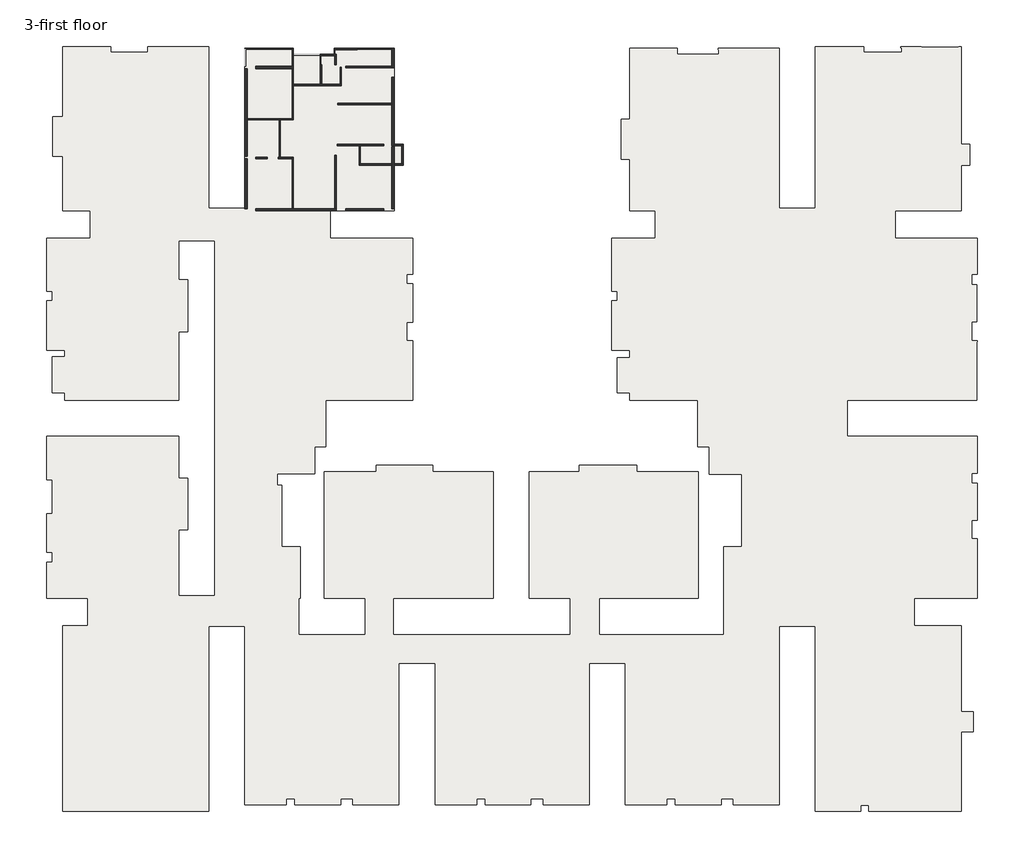
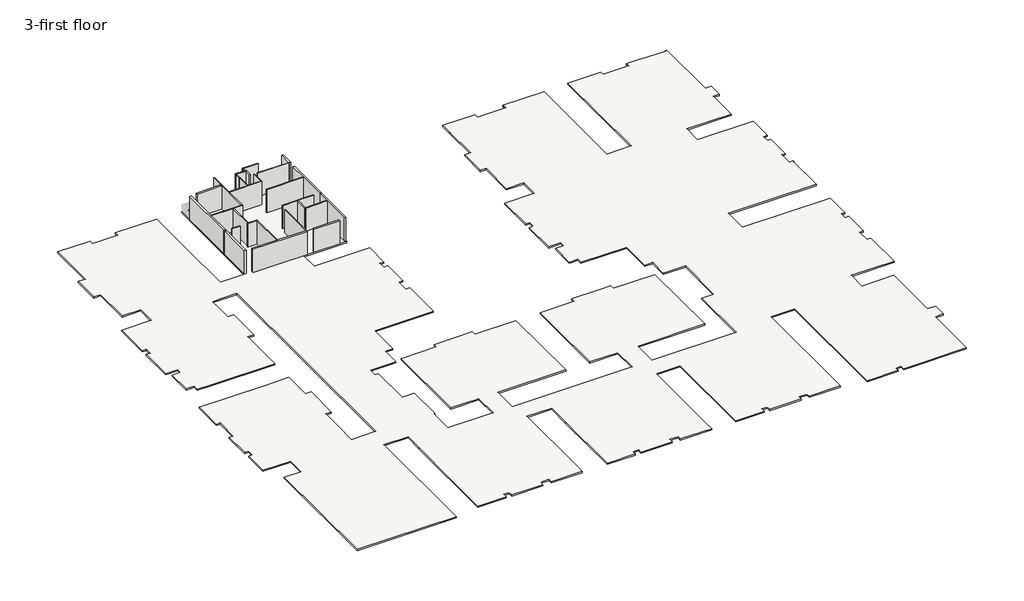
# One storey, part 1 of 2: 32 walls, 1 slab.
"""IFC4 building model written with IfcOpenShell, lengths in millimetres."""

from ifc_helpers import new_model, si_unit, frame, origin, place, context, project, spatial, polyline, outline, extrude, faceted_brep, element, save

model = new_model("IFC4")

# Units and contexts
model_context = context("Model", 3, world=origin())
ifc_project = project(units=[si_unit("LENGTHUNIT", "METRE", prefix="MILLI")], contexts=[model_context])

# Site, building, storey
site = spatial("IfcSite", under=ifc_project)
building = spatial("IfcBuilding", under=site)
storey = spatial("IfcBuildingStorey", under=building, Name="3-first floor", Elevation=3505.2)

# Slab
placement = place(None, origin())
element("IfcSlab", 1, ObjectType="6\" floor", at=placement, inside=storey, context=model_context, shape_type="SweptSolid", body=[
    extrude(outline(polyline([(-40067.5946761, 34417.793059), (-40067.5946761, 36703.793059), (-42359.0159175, 36703.793059), (-42359.0159175, 41288.4930592), (-43200.0473754, 41288.4930592), (-43200.0473754, 44641.2930588), (-42359.0159175, 44641.2930588), (-42359.0159175, 50522.1625405), (-38355.6844598, 50522.1625405), (-38355.6844598, 50026.0999818), (-35221.6159175, 50026.0999818), (-35221.6159175, 50522.1625405), (-30090.8159175, 50522.1625405), (-30090.8159175, 44272.6043046), (-30090.8159175, 36920.6122854), (-27080.9159175, 36920.6122854), (-27080.9159175, 50369.7625405), (-23004.2159175, 50369.7625405), (-23004.2159175, 49873.6841178), (-19562.5159175, 49873.6841178), (-19562.5159175, 50369.7625405), (-14510.7473752, 50369.7625405), (-14510.7473752, 42291.793059), (-13786.847376, 42291.793059), (-13786.847376, 40564.593059), (-14510.7473752, 40564.593059), (-14510.7473752, 39345.393059), (-14510.7473752, 36703.793059), (-19901.4109088, 36703.793059), (-19901.4109088, 34417.793059), (-12985.9778949, 34417.793059), (-12985.9778949, 31382.4930587), (-13482.0473762, 31382.4930587), (-13482.0473762, 30582.3930587), (-12985.9778949, 30582.3930587), (-12985.9778949, 27342.8846057), (-13482.047376, 27342.8846057), (-13482.047376, 25819.8930592), (-12985.9778949, 25819.8930592), (-12985.9778949, 20790.6930592), (-20261.0159173, 20790.6930592), (-20261.0159173, 16904.4930621), (-21213.5159173, 16904.4930621), (-21213.5159173, 14605.7930651), (-24363.1159173, 14605.7930651), (-24363.1159173, 13640.5930617), (-23956.7159173, 13640.5930617), (-23956.7159173, 8484.3930618), (-22432.7159173, 8484.3930618), (-22432.7159173, 4153.6930617), (-22552.879451, 4153.6930617), (-22552.879451, 1105.693062), (-16952.179451, 1105.693062), (-16952.179451, 4153.693062), (-20419.279451, 4153.693062), (-20419.279451, 14808.993062), (-16050.479451, 14808.993062), (-16050.479451, 15342.393062), (-11287.979451, 15342.393062), (-11287.979451, 14808.993062), (-6207.979451, 14808.993062), (-6207.979451, 4153.693062), (-14589.979451, 4153.693062), (-14589.979451, 1105.693062), (269.020549, 1105.693062), (269.020549, 4153.693062), (-3198.079451, 4153.693062), (-3198.079451, 11358.3599187), (-3198.079451, 14808.993062), (56.8139168, 14808.993062), (1031.020549, 14808.993062), (1031.020549, 15342.393062), (4447.320549, 15342.393062), (5844.320549, 15342.393062), (5844.320549, 14808.993062), (11013.220549, 14808.993062), (11013.220549, 4153.693062), (2707.420549, 4153.693062), (2707.420549, 1105.693062), (13149.6520067, 1105.693062), (13149.6520067, 8509.7930618), (14673.6520067, 8509.7930618), (14673.6520067, 14580.393062), (11930.4520067, 14580.393062), (11930.4520067, 16904.493062), (10977.9520067, 16904.493062), (10977.9520067, 20790.6930623), (5260.120549, 20790.6930623), (5260.120549, 21438.3930622), (4231.4205485, 21438.3930622), (4231.4205485, 24372.093062), (5260.120549, 24372.093062), (5260.120549, 25007.093059), (3735.3510676, 25007.093059), (3735.3510676, 29155.9725232), (4231.4205489, 29155.9725232), (4231.4205489, 29972.793059), (3735.3510673, 29972.793059), (3735.3510673, 34417.793062), (7406.6788707, 34417.793062), (7406.6788707, 36703.793062), (5262.3642609, 36703.793062), (5262.3642609, 41072.593062), (4538.4642607, 41072.593062), (4538.4642607, 44425.393062), (5262.3642609, 44425.393062), (5262.3642609, 48850.8834653), (5262.3642609, 50369.7625405), (9260.0328033, 50369.7625405), (9260.0328033, 49861.0033239), (12752.53262, 49861.0033239), (12752.53262, 50255.4613897), (12701.7328035, 50255.4613897), (12701.7328035, 50369.7625391), (17833.6918765, 50369.7625391), (17833.6918765, 36920.6122884), (20843.020549, 36920.6122884), (20843.020549, 50522.1625435), (24922.5520067, 50522.1625435), (24922.5520067, 50026.0682305), (28107.4205486, 50026.0682305), (28107.4205486, 50407.8625436), (28056.620549, 50407.8625436), (28056.620549, 50522.1625436), (29758.420549, 50522.1625436), (29758.420549, 50464.6477108), (32908.0205485, 50464.6477108), (32908.0205485, 50522.1625436), (33111.220549, 50522.1625436), (33111.220549, 42291.793059), (33835.1205481, 42291.793059), (33835.1205481, 40564.593059), (33111.220549, 40564.593059), (33111.220549, 36703.793062), (27583.8962522, 36703.793062), (27583.8962522, 34417.793062), (34483.5900291, 34417.793062), (34483.5900291, 31369.7930587), (33987.5205478, 31369.7930587), (33987.5205478, 30518.8930587), (34420.0900291, 30518.8930587), (34420.0900291, 27393.6846085), (33987.520548, 27393.6846085), (33987.520548, 25819.8930599), (34483.5900268, 25819.8930599), (34483.5900268, 25718.293062), (34420.0900291, 25718.293062), (34420.0900291, 20790.6930621), (23560.820549, 20790.6930621), (23560.820549, 17780.7930626), (34470.8900301, 17780.7930626), (34470.8900301, 14669.2930621), (33987.5205488, 14669.2930621), (33987.5205488, 13831.5086417), (34470.8900301, 13831.5086417), (34470.8900301, 10719.5930626), (33987.520549, 10719.5930626), (33987.520549, 9144.7930626), (34483.5900287, 9144.7930626), (34483.5900287, 4153.6930626), (29171.7035804, 4153.6930626), (29171.7035804, 1867.6930615), (33111.220549, 1867.6930615), (33111.220549, -4382.5255151), (33111.220549, -5358.6069385), (34139.9205493, -5358.6069385), (34139.9205493, -7035.0069385), (33111.220549, -7035.0069385), (33111.220549, -12216.6069385), (33111.220549, -13741.3764277), (25342.0873109, -13741.3764277), (25342.0873109, -13245.3069411), (24664.0464127, -13245.3069411), (24664.0464127, -13741.3764224), (20843.020549, -13741.3764224), (20843.020549, 1791.493062), (17833.120549, 1791.493062), (17833.1205601, -12469.7116346), (17833.1205601, -13181.806941), (13972.320549, -13181.806941), (13972.320549, -12686.5069412), (12968.4328031, -12686.5069412), (12968.4328031, -13181.806941), (9079.9890911, -13181.806941), (9079.9890911, -12686.5069411), (8371.620549, -12686.5069411), (8371.620549, -13181.806941), (4879.120549, -13181.806941), (4879.120549, -1281.906938), (1869.220549, -1281.906938), (1869.2205601, -11657.8069405), (1869.2205601, -13181.806941), (-1991.579451, -13181.806941), (-1991.579451, -12686.5069412), (-3032.979451, -12686.5069412), (-3032.979451, -13181.806941), (-6883.9109089, -13181.806941), (-6883.9109089, -12686.5069411), (-7592.2794511, -12686.5069411), (-7592.2794511, -13181.806941), (-11084.779451, -13181.806941), (-11084.779451, -4364.4278939), (-11084.779451, -1281.906938), (-14132.779451, -1281.906938), (-14132.7794399, -11657.8069405), (-14132.7794399, -13181.806941), (-17993.579451, -13181.806941), (-17993.579451, -12686.5069412), (-19034.979451, -12686.5069412), (-19034.979451, -13181.806941), (-22885.9109089, -13181.806941), (-22885.9109089, -12686.5069411), (-23594.279451, -12686.5069411), (-23594.279451, -13181.806941), (-27086.779451, -13181.806941), (-27086.779451, -630.8240429), (-27086.779451, 1791.493062), (-30096.679451, 1791.493062), (-30096.679451, -13741.3764224), (-42359.0159175, -13741.3764224), (-42359.0159175, 1867.6930615), (-40274.4710752, 1867.6930615), (-40274.4710752, 4153.6930619), (-43737.2489325, 4153.6930619), (-43737.2489325, 7188.9930625), (-43244.0109091, 7188.9930625), (-43244.0109091, 8035.7406725), (-43740.0803903, 8035.7406725), (-43740.0803903, 11278.3930621), (-43244.0109091, 11278.3930621), (-43244.0109091, 14123.1930621), (-43737.2489325, 14123.1930621), (-43737.2489325, 17780.7930616), (-35451.4646582, 17780.7930627), (-32611.279451, 17780.7930627), (-32611.279451, 14237.4930616), (-31890.2109088, 14237.4930616), (-31890.2109088, 9905.7846088), (-32611.2794515, 9905.7846088), (-32611.279451, 7112.7930625), (-32611.279451, 4382.2930626), (-29601.379451, 4382.2930626), (-29601.379451, 34189.193059), (-32614.110909, 34189.193059), (-32614.110909, 32865.9503102), (-32614.110909, 30913.6015126), (-31890.210909, 30913.6015126), (-31890.210909, 27445.4930592), (-31890.210909, 26569.1930592), (-32614.110909, 26569.1930592), (-32614.110909, 20790.6930591), (-40664.490635, 20790.6930591), (-42212.479451, 20790.6930591), (-42212.479451, 21438.393059), (-43244.0109092, 21438.393059), (-43244.0109092, 24435.5930825), (-42215.3109116, 24435.5930825), (-42215.3109116, 24994.393059), (-43740.0803903, 24994.393059), (-43740.0803903, 29172.693059), (-43244.0109091, 29172.693059), (-43244.0109091, 29972.793059), (-43740.0803903, 29972.793059), (-43740.0803903, 34417.793059), (-40067.5946761, 34417.793059)])), frame((0.0, 0.0, 3352.8), z_axis=(0.0, 0.0, 1.0), x_axis=(1.0, 0.0, 0.0)), (0.0, 0.0, 1.0), 152.4),
])

# Walls
element("IfcWall", 2, ObjectType="1\"", at=placement, inside=storey, context=model_context, shape_type="SweptSolid", body=[
    extrude(outline(polyline([(-20680.9533155, 49759.3844575), (-20680.9533155, 49003.2834458), (-20721.5933155, 49003.2834458), (-20721.5933155, 49759.3844575), (-20680.9533155, 49759.3844575)])), frame((0.0, 0.0, 3505.2), z_axis=(0.0, 0.0, 1.0), x_axis=(1.0, 0.0, 0.0)), (0.0, 0.0, 1.0), 3048.0),
])
element("IfcWall", 3, ObjectType="2.5\"", at=placement, inside=storey, context=model_context, shape_type="SweptSolid", body=[
    extrude(outline(polyline([(-19562.5159175, 49873.6844575), (-19562.5159175, 50255.4625405), (-19504.0959175, 50255.4625405), (-19504.0959175, 49873.6844575), (-19562.5159175, 49873.6844575)])), frame((0.0, 0.0, 3505.2), z_axis=(0.0, 0.0, 1.0), x_axis=(1.0, 0.0, 0.0)), (0.0, 0.0, 1.0), 3048.0),
])
element("IfcWall", 4, ObjectType="4\" wall", at=placement, inside=storey, context=model_context, shape_type="Brep", body=[
    faceted_brep([(-26877.7159175, 44361.8930595, 3505.2), (-24198.0159175, 44361.8930595, 3505.2), (-24096.4159175, 44361.8930595, 3505.2), (-23004.2159175, 44361.8930595, 3505.2), (-23004.2159175, 44361.8930595, 6553.2), (-24096.4159175, 44361.8930595, 6553.2), (-24198.0159175, 44361.8930595, 6553.2), (-26877.7159175, 44361.8930595, 6553.2), (-26877.7159175, 44463.4930595, 3505.2), (-26877.7159175, 44463.4930595, 6553.2), (-23105.8159175, 44463.4930595, 6553.2), (-23004.2159175, 44463.4930595, 6553.2), (-23004.2159175, 44463.4930595, 3505.2), (-23105.8159175, 44463.4930595, 3505.2)], [[[0, 1, 2, 3, 4, 5, 6, 7]], [[8, 9, 10, 11, 12, 13]], [[3, 2, 1, 0, 8, 13, 12]], [[7, 6, 5, 4, 11, 10, 9]], [[0, 7, 9, 8]], [[4, 3, 12, 11]]]),
])
element("IfcWall", 5, ObjectType="4\" wall", at=placement, inside=storey, context=model_context, shape_type="Brep", body=[
    faceted_brep([(-23004.2159175, 44463.4930595, 3505.2), (-23004.2159175, 47237.9834458, 3505.2), (-23004.2159175, 47339.5834458, 3505.2), (-23004.2159175, 48647.683515, 3505.2), (-23004.2159175, 48647.683515, 6553.2), (-23004.2159175, 47339.5834458, 6553.2), (-23004.2159175, 47237.9834458, 6553.2), (-23004.2159175, 44463.4930595, 6553.2), (-23105.8159175, 44463.4930595, 3505.2), (-23105.8159175, 44463.4930595, 6553.2), (-23105.8159175, 48647.683515, 6553.2), (-23105.8159175, 48647.683515, 3505.2)], [[[0, 1, 2, 3, 4, 5, 6, 7]], [[8, 9, 10, 11]], [[3, 2, 1, 0, 8, 11]], [[7, 6, 5, 4, 10, 9]], [[0, 7, 9, 8]], [[4, 3, 11, 10]]]),
])
element("IfcWall", 6, ObjectType="4\" wall", at=placement, inside=storey, context=model_context, shape_type="Brep", body=[
    faceted_brep([(-20731.7533155, 49003.2834458, 3505.2), (-20731.7533155, 47339.5834458, 3505.2), (-20731.7533155, 47339.5834458, 6553.2), (-20731.7533155, 49003.2834458, 6553.2), (-20630.1533155, 49003.2834458, 3505.2), (-20630.1533155, 49003.2834458, 6553.2), (-20630.1533155, 47339.5834458, 6553.2), (-20630.1533155, 47339.5834458, 3505.2), (-20721.5933155, 49003.2834458, 3505.2), (-20680.9533155, 49003.2834458, 3505.2), (-20680.9533155, 49003.2834458, 6553.2), (-20721.5933155, 49003.2834458, 6553.2)], [[[0, 1, 2, 3]], [[4, 5, 6, 7]], [[1, 0, 8, 9, 4, 7]], [[3, 2, 6, 5, 10, 11]], [[0, 3, 11, 10, 5, 4, 9, 8]], [[2, 1, 7, 6]]]),
])
element("IfcWall", 7, ObjectType="4\" wall", at=placement, inside=storey, context=model_context, shape_type="Brep", body=[
    faceted_brep([(-23004.2159175, 47237.9834458, 3505.2), (-18955.7473752, 47237.9834458, 3505.2), (-18955.7473752, 47237.9834458, 6553.2), (-23004.2159175, 47237.9834458, 6553.2), (-23004.2159175, 47339.5834458, 3505.2), (-23004.2159175, 47339.5834458, 6553.2), (-20731.7533155, 47339.5834458, 6553.2), (-20630.1533155, 47339.5834458, 6553.2), (-19057.3473752, 47339.5834458, 6553.2), (-18955.7473752, 47339.5834458, 6553.2), (-18955.7473752, 47339.5834458, 3505.2), (-19057.3473752, 47339.5834458, 3505.2), (-20630.1533155, 47339.5834458, 3505.2), (-20731.7533155, 47339.5834458, 3505.2)], [[[0, 1, 2, 3]], [[4, 5, 6, 7, 8, 9, 10, 11, 12, 13]], [[1, 0, 4, 13, 12, 11, 10]], [[3, 2, 9, 8, 7, 6, 5]], [[2, 1, 10, 9]], [[0, 3, 5, 4]]]),
])
element("IfcWall", 8, ObjectType="4\" wall", at=placement, inside=storey, context=model_context, shape_type="SweptSolid", body=[
    extrude(outline(polyline([(-18955.7473752, 48800.0834491), (-18955.7473752, 47339.5834458), (-19057.3473752, 47339.5834458), (-19057.3473752, 48800.0834491), (-18955.7473752, 48800.0834491)])), frame((0.0, 0.0, 3505.2), z_axis=(0.0, 0.0, 1.0), x_axis=(1.0, 0.0, 0.0)), (0.0, 0.0, 1.0), 3048.0),
])
element("IfcWall", 9, ObjectType="4\" wall", at=placement, inside=storey, context=model_context, shape_type="SweptSolid", body=[
    extrude(outline(polyline([(-18587.4473751, 48850.8834491), (-14713.9473752, 48850.8834491), (-14713.9473752, 48749.2834491), (-18587.4473751, 48749.2834491), (-18587.4473751, 48850.8834491)])), frame((0.0, 0.0, 3505.2), z_axis=(0.0, 0.0, 1.0), x_axis=(1.0, 0.0, 0.0)), (0.0, 0.0, 1.0), 3048.0),
])
element("IfcWall", 10, ObjectType="4\" wall", at=placement, inside=storey, context=model_context, shape_type="SweptSolid", body=[
    extrude(outline(polyline([(-19285.9473752, 45746.193059), (-14713.9473752, 45746.193059), (-14713.9473752, 45644.593059), (-19285.9473752, 45644.593059), (-19285.9473752, 45746.193059)])), frame((0.0, 0.0, 3505.2), z_axis=(0.0, 0.0, 1.0), x_axis=(1.0, 0.0, 0.0)), (0.0, 0.0, 1.0), 3048.0),
])
element("IfcWall", 11, ObjectType="4\" wall", at=placement, inside=storey, context=model_context, shape_type="Brep", body=[
    faceted_brep([(-15425.1473762, 42291.793059, 3505.2), (-19298.6473752, 42291.793059, 3505.2), (-19298.6473752, 42291.793059, 6553.2), (-15425.1473762, 42291.793059, 6553.2), (-15425.1473762, 42190.193059, 3505.2), (-15425.1473762, 42190.193059, 6553.2), (-17380.9473752, 42190.193059, 6553.2), (-17482.5473752, 42190.193059, 6553.2), (-19298.6473752, 42190.193059, 6553.2), (-19298.6473752, 42190.193059, 3505.2), (-17482.5473752, 42190.193059, 3505.2), (-17380.9473752, 42190.193059, 3505.2)], [[[0, 1, 2, 3]], [[4, 5, 6, 7, 8, 9, 10, 11]], [[1, 0, 4, 11, 10, 9]], [[2, 1, 9, 8]], [[3, 2, 8, 7, 6, 5]], [[0, 3, 5, 4]]]),
])
element("IfcWall", 12, ObjectType="4\" wall", at=placement, inside=storey, context=model_context, shape_type="SweptSolid", body=[
    extrude(outline(polyline([(-19501.8473752, 36906.993059), (-19501.8473752, 41377.3930622), (-19400.2473752, 41377.3930622), (-19400.2473752, 36906.993059), (-19501.8473752, 36906.993059)])), frame((0.0, 0.0, 3505.2), z_axis=(0.0, 0.0, 1.0), x_axis=(1.0, 0.0, 0.0)), (0.0, 0.0, 1.0), 3048.0),
])
element("IfcWall", 13, ObjectType="4\" wall", at=placement, inside=storey, context=model_context, shape_type="Brep", body=[
    faceted_brep([(-17482.5473752, 42190.193059, 3505.2), (-17482.5473752, 40564.593059, 3505.2), (-17482.5473752, 40564.593059, 6553.2), (-17482.5473752, 42190.193059, 6553.2), (-17380.9473752, 42190.193059, 3505.2), (-17380.9473752, 42190.193059, 6553.2), (-17380.9473752, 40666.193059, 6553.2), (-17380.9473752, 40564.593059, 6553.2), (-17380.9473752, 40564.593059, 3505.2), (-17380.9473752, 40666.193059, 3505.2)], [[[0, 1, 2, 3]], [[4, 5, 6, 7, 8, 9]], [[1, 0, 4, 9, 8]], [[3, 2, 7, 6, 5]], [[0, 3, 5, 4]], [[2, 1, 8, 7]]]),
])
element("IfcWall", 14, ObjectType="4\" wall", at=placement, inside=storey, context=model_context, shape_type="SweptSolid", body=[
    extrude(outline(polyline([(-14713.9473762, 40564.593059), (-17380.9473752, 40564.593059), (-17380.9473752, 40666.193059), (-14713.9473762, 40666.193059), (-14713.9473762, 40564.593059)])), frame((0.0, 0.0, 3505.2), z_axis=(0.0, 0.0, 1.0), x_axis=(1.0, 0.0, 0.0)), (0.0, 0.0, 1.0), 3048.0),
])
element("IfcWall", 15, ObjectType="4\" wall", at=placement, inside=storey, context=model_context, shape_type="Brep", body=[
    faceted_brep([(-14510.7473762, 40564.593059, 3505.2), (-13786.847376, 40564.593059, 3505.2), (-13786.847376, 40564.593059, 5334.0), (-14510.7473762, 40564.593059, 5334.0), (-14510.7473762, 40666.193059, 3505.2), (-14510.7473762, 40666.193059, 5334.0), (-13888.447376, 40666.193059, 5334.0), (-13786.847376, 40666.193059, 5334.0), (-13786.847376, 40666.193059, 3505.2), (-13888.447376, 40666.193059, 3505.2)], [[[0, 1, 2, 3]], [[4, 5, 6, 7, 8, 9]], [[1, 0, 4, 9, 8]], [[3, 2, 7, 6, 5]], [[0, 3, 5, 4]], [[2, 1, 8, 7]]]),
])
element("IfcWall", 16, ObjectType="4\" wall", at=placement, inside=storey, context=model_context, shape_type="Brep", body=[
    faceted_brep([(-14510.7473752, 42190.193059, 3505.2), (-13888.447376, 42190.193059, 3505.2), (-13786.847376, 42190.193059, 3505.2), (-13786.847376, 42190.193059, 5334.0), (-13888.447376, 42190.193059, 5334.0), (-14510.7473752, 42190.193059, 5334.0), (-14510.7473752, 42291.793059, 3505.2), (-14510.7473752, 42291.793059, 5334.0), (-13786.847376, 42291.793059, 5334.0), (-13786.847376, 42291.793059, 3505.2)], [[[0, 1, 2, 3, 4, 5]], [[6, 7, 8, 9]], [[2, 1, 0, 6, 9]], [[5, 4, 3, 8, 7]], [[0, 5, 7, 6]], [[3, 2, 9, 8]]]),
])
element("IfcWall", 17, ObjectType="4\" wall", at=placement, inside=storey, context=model_context, shape_type="SweptSolid", body=[
    extrude(outline(polyline([(-13888.447376, 40666.193059), (-13888.447376, 42190.193059), (-13786.847376, 42190.193059), (-13786.847376, 40666.193059), (-13888.447376, 40666.193059)])), frame((0.0, 0.0, 3505.2), z_axis=(0.0, 0.0, 1.0), x_axis=(1.0, 0.0, 0.0)), (0.0, 0.0, 1.0), 1828.8),
])
element("IfcWall", 18, ObjectType="4\" wall", at=placement, inside=storey, context=model_context, shape_type="Brep", body=[
    faceted_brep([(-23004.2159175, 36906.993059, 3505.2), (-23004.2159175, 41212.293059, 3505.2), (-23004.2159175, 41212.293059, 6553.2), (-23004.2159175, 36906.993059, 6553.2), (-23105.8159175, 36906.993059, 3505.2), (-23105.8159175, 36906.993059, 6553.2), (-23105.8159175, 41110.693059, 6553.2), (-23105.8159175, 41212.293059, 6553.2), (-23105.8159175, 41212.293059, 3505.2), (-23105.8159175, 41110.693059, 3505.2)], [[[0, 1, 2, 3]], [[4, 5, 6, 7, 8, 9]], [[1, 0, 4, 9, 8]], [[3, 2, 7, 6, 5]], [[0, 3, 5, 4]], [[2, 1, 8, 7]]]),
])
element("IfcWall", 19, ObjectType="4\" wall", at=placement, inside=storey, context=model_context, shape_type="Brep", body=[
    faceted_brep([(-23105.8159175, 41212.293059, 3505.2), (-24096.4159175, 41212.293059, 3505.2), (-24198.0159175, 41212.293059, 3505.2), (-24261.5159175, 41212.293059, 3505.2), (-24261.5159175, 41212.293059, 6553.2), (-24198.0159175, 41212.293059, 6553.2), (-24096.4159175, 41212.293059, 6553.2), (-23105.8159175, 41212.293059, 6553.2), (-23105.8159175, 41110.693059, 3505.2), (-23105.8159175, 41110.693059, 6553.2), (-24261.5159175, 41110.693059, 6553.2), (-24261.5159175, 41110.693059, 3505.2)], [[[0, 1, 2, 3, 4, 5, 6, 7]], [[8, 9, 10, 11]], [[3, 2, 1, 0, 8, 11]], [[4, 3, 11, 10]], [[7, 6, 5, 4, 10, 9]], [[0, 7, 9, 8]]]),
])
element("IfcWall", 20, ObjectType="4\" wall", at=placement, inside=storey, context=model_context, shape_type="SweptSolid", body=[
    extrude(outline(polyline([(-26166.5159175, 41212.293059), (-25175.9159175, 41212.293059), (-25175.9159175, 41110.693059), (-26166.5159175, 41110.693059), (-26166.5159175, 41212.293059)])), frame((0.0, 0.0, 3505.2), z_axis=(0.0, 0.0, 1.0), x_axis=(1.0, 0.0, 0.0)), (0.0, 0.0, 1.0), 3048.0),
])
element("IfcWall", 21, ObjectType="4\" wall", at=placement, inside=storey, context=model_context, shape_type="SweptSolid", body=[
    extrude(outline(polyline([(-24096.4159175, 44361.8930595), (-24096.4159175, 41212.293059), (-24198.0159175, 41212.293059), (-24198.0159175, 44361.8930595), (-24096.4159175, 44361.8930595)])), frame((0.0, 0.0, 3505.2), z_axis=(0.0, 0.0, 1.0), x_axis=(1.0, 0.0, 0.0)), (0.0, 0.0, 1.0), 3048.0),
])
element("IfcWall", 22, ObjectType="4\" wall", at=placement, inside=storey, context=model_context, shape_type="SweptSolid", body=[
    extrude(outline(polyline([(-23105.8159175, 48850.883515), (-23105.8159175, 50369.7625405), (-23004.2159175, 50369.7625405), (-23004.2159175, 48850.883515), (-23105.8159175, 48850.883515)])), frame((0.0, 0.0, 3505.2), z_axis=(0.0, 0.0, 1.0), x_axis=(1.0, 0.0, 0.0)), (0.0, 0.0, 1.0), 3048.0),
])
element("IfcWall", 23, ObjectType="4\" wall", at=placement, inside=storey, context=model_context, shape_type="SweptSolid", body=[
    extrude(outline(polyline([(-19501.8473751, 49003.2834458), (-19501.8473751, 49759.3844575), (-19400.2473751, 49759.3844575), (-19400.2473751, 49003.2834458), (-19501.8473751, 49003.2834458)])), frame((0.0, 0.0, 3505.2), z_axis=(0.0, 0.0, 1.0), x_axis=(1.0, 0.0, 0.0)), (0.0, 0.0, 1.0), 3048.0),
])
element("IfcWall", 24, ObjectType="4.5\" wall", at=placement, inside=storey, context=model_context, shape_type="Brep", body=[
    faceted_brep([(-19400.2473751, 49873.6844575, 3505.2), (-19504.0959175, 49873.6844575, 3505.2), (-19562.5159175, 49873.6844575, 3505.2), (-20721.5933155, 49873.6844575, 3505.2), (-20721.5933155, 49873.6844575, 6553.2), (-19562.5159175, 49873.6844575, 6553.2), (-19504.0959175, 49873.6844575, 6553.2), (-19400.2473751, 49873.6844575, 6553.2), (-19400.2473751, 49759.3844575, 3505.2), (-19400.2473751, 49759.3844575, 6553.2), (-19501.8473751, 49759.3844575, 6553.2), (-20680.9533155, 49759.3844575, 6553.2), (-20721.5933155, 49759.3844575, 6553.2), (-20721.5933155, 49759.3844575, 3505.2), (-20680.9533155, 49759.3844575, 3505.2), (-19501.8473751, 49759.3844575, 3505.2)], [[[0, 1, 2, 3, 4, 5, 6, 7]], [[8, 9, 10, 11, 12, 13, 14, 15]], [[3, 2, 1, 0, 8, 15, 14, 13]], [[7, 6, 5, 4, 12, 11, 10, 9]], [[0, 7, 9, 8]], [[4, 3, 13, 12]]]),
])
element("IfcWall", 25, ObjectType="4.5\" wall", at=placement, inside=storey, context=model_context, shape_type="Brep", body=[
    faceted_brep([(-17647.6473751, 50369.7625405, 3505.2), (-19562.5159175, 50369.7625405, 3505.2), (-19562.5159175, 50369.7625405, 6553.2), (-17647.6473751, 50369.7625405, 6553.2), (-17647.6473751, 50255.4625405, 3505.2), (-17647.6473751, 50255.4625405, 6553.2), (-19504.0959175, 50255.4625405, 6553.2), (-19562.5159175, 50255.4625405, 6553.2), (-19562.5159175, 50255.4625405, 3505.2), (-19504.0959175, 50255.4625405, 3505.2)], [[[0, 1, 2, 3]], [[4, 5, 6, 7, 8, 9]], [[1, 0, 4, 9, 8]], [[3, 2, 7, 6, 5]], [[0, 3, 5, 4]], [[2, 1, 8, 7]]]),
])
element("IfcWall", 26, ObjectType="8\" wall", at=placement, inside=storey, context=model_context, shape_type="Brep", body=[
    faceted_brep([(-14713.9473752, 50369.7625405, 3505.2), (-14713.9473752, 48850.8834491, 3505.2), (-14713.9473752, 48749.2834491, 3505.2), (-14713.9473752, 48749.2834491, 6553.2), (-14713.9473752, 48850.8834491, 6553.2), (-14713.9473752, 50369.7625405, 6553.2), (-14510.7473752, 50369.7625405, 3505.2), (-14510.7473752, 50369.7625405, 6553.2), (-14510.7473752, 48850.8834491, 6553.2), (-14510.7473752, 48749.2834491, 6553.2), (-14510.7473752, 48749.2834491, 3505.2), (-14510.7473752, 48850.8834491, 3505.2)], [[[0, 1, 2, 3, 4, 5]], [[6, 7, 8, 9, 10, 11]], [[2, 1, 0, 6, 11, 10]], [[5, 4, 3, 9, 8, 7]], [[0, 5, 7, 6]], [[3, 2, 10, 9]]]),
])
element("IfcWall", 27, ObjectType="8\" wall", at=placement, inside=storey, context=model_context, shape_type="Brep", body=[
    faceted_brep([(-14713.9473752, 47936.4834491, 3505.2), (-14713.9473752, 45746.193059, 3505.2), (-14713.9473752, 45644.593059, 3505.2), (-14713.9473752, 42291.793059, 3505.2), (-14713.9473752, 42190.193059, 3505.2), (-14713.9473752, 42190.193059, 6553.2), (-14713.9473752, 42291.793059, 6553.2), (-14713.9473752, 45644.593059, 6553.2), (-14713.9473752, 45746.193059, 6553.2), (-14713.9473752, 47936.4834491, 6553.2), (-14510.7473752, 47936.4834491, 3505.2), (-14510.7473752, 47936.4834491, 6553.2), (-14510.7473752, 42190.193059, 6553.2), (-14510.7473752, 42190.193059, 5334.0), (-14510.7473752, 42190.193059, 3505.2), (-14510.7473752, 42291.793059, 3505.2)], [[[0, 1, 2, 3, 4, 5, 6, 7, 8, 9]], [[10, 11, 12, 13, 14, 15]], [[4, 3, 2, 1, 0, 10, 15, 14]], [[9, 8, 7, 6, 5, 12, 11]], [[0, 9, 11, 10]], [[5, 4, 14, 13, 12]]]),
])
element("IfcWall", 28, ObjectType="8\" wall", at=placement, inside=storey, context=model_context, shape_type="Brep", body=[
    faceted_brep([(-26166.5159189, 48647.683515, 3505.2), (-23105.8159175, 48647.683515, 3505.2), (-23004.2159175, 48647.683515, 3505.2), (-23004.2159175, 48647.683515, 6553.2), (-23105.8159175, 48647.683515, 6553.2), (-26166.5159189, 48647.683515, 6553.2), (-26166.5159189, 48850.883515, 3505.2), (-26166.5159189, 48850.883515, 6553.2), (-23105.8159175, 48850.883515, 6553.2), (-23004.2159175, 48850.883515, 6553.2), (-23004.2159175, 48850.883515, 3505.2), (-23105.8159175, 48850.883515, 3505.2)], [[[0, 1, 2, 3, 4, 5]], [[6, 7, 8, 9, 10, 11]], [[2, 1, 0, 6, 11, 10]], [[5, 4, 3, 9, 8, 7]], [[0, 5, 7, 6]], [[3, 2, 10, 9]]]),
])
element("IfcWall", 29, ObjectType="8\" wall", at=placement, inside=storey, context=model_context, shape_type="Brep", body=[
    faceted_brep([(-27080.9159175, 48647.683515, 3505.2), (-27080.9159175, 41313.8930626, 3505.2), (-27080.9159175, 41313.8930626, 6553.2), (-27080.9159175, 48647.683515, 6553.2), (-26877.7159175, 48647.683515, 3505.2), (-26877.7159175, 48647.683515, 6553.2), (-26877.7159175, 44463.4930595, 6553.2), (-26877.7159175, 44361.8930595, 6553.2), (-26877.7159175, 41313.8930626, 6553.2), (-26877.7159175, 41313.8930626, 3505.2), (-26877.7159175, 44361.8930595, 3505.2), (-26877.7159175, 44463.4930595, 3505.2)], [[[0, 1, 2, 3]], [[4, 5, 6, 7, 8, 9, 10, 11]], [[1, 0, 4, 11, 10, 9]], [[2, 1, 9, 8]], [[3, 2, 8, 7, 6, 5]], [[0, 3, 5, 4]]]),
])
element("IfcWall", 30, ObjectType="8\" wall", at=placement, inside=storey, context=model_context, shape_type="SweptSolid", body=[
    extrude(outline(polyline([(-27080.9159175, 36906.993059), (-27080.9159175, 41110.6930626), (-26877.7159175, 41110.6930626), (-26877.7159175, 36906.993059), (-27080.9159175, 36906.993059)])), frame((0.0, 0.0, 3505.2), z_axis=(0.0, 0.0, 1.0), x_axis=(1.0, 0.0, 0.0)), (0.0, 0.0, 1.0), 3048.0),
])
element("IfcWall", 31, ObjectType="8\" wall", at=placement, inside=storey, context=model_context, shape_type="Brep", body=[
    faceted_brep([(-26166.5159175, 36703.793059, 3505.2), (-19501.8473751, 36703.793059, 3505.2), (-19400.2473752, 36703.793059, 3505.2), (-19400.2473752, 36703.793059, 6553.2), (-19501.8473751, 36703.793059, 6553.2), (-26166.5159175, 36703.793059, 6553.2), (-26166.5159175, 36906.993059, 3505.2), (-26166.5159175, 36906.993059, 6553.2), (-23105.8159175, 36906.993059, 6553.2), (-23004.2159175, 36906.993059, 6553.2), (-19501.8473752, 36906.993059, 6553.2), (-19400.2473752, 36906.993059, 6553.2), (-19400.2473752, 36906.993059, 3505.2), (-19501.8473752, 36906.993059, 3505.2), (-23004.2159175, 36906.993059, 3505.2), (-23105.8159175, 36906.993059, 3505.2)], [[[0, 1, 2, 3, 4, 5]], [[6, 7, 8, 9, 10, 11, 12, 13, 14, 15]], [[2, 1, 0, 6, 15, 14, 13, 12]], [[5, 4, 3, 11, 10, 9, 8, 7]], [[0, 5, 7, 6]], [[3, 2, 12, 11]]]),
])
element("IfcWall", 32, ObjectType="8\" wall", at=placement, inside=storey, context=model_context, shape_type="Brep", body=[
    faceted_brep([(-14713.9473762, 42088.593059, 3505.2), (-14713.9473762, 40666.193059, 3505.2), (-14713.9473762, 40564.593059, 3505.2), (-14713.9473762, 36906.993059, 3505.2), (-14713.9473762, 36906.993059, 6553.2), (-14713.9473762, 40564.593059, 6553.2), (-14713.9473762, 40666.193059, 6553.2), (-14713.9473762, 42088.593059, 6553.2), (-14510.7473762, 42088.593059, 3505.2), (-14510.7473762, 42088.593059, 6553.2), (-14510.7473762, 36906.993059, 6553.2), (-14510.7473762, 36906.993059, 3505.2), (-14510.7473762, 40564.593059, 3505.2), (-14510.7473762, 40666.193059, 3505.2)], [[[0, 1, 2, 3, 4, 5, 6, 7]], [[8, 9, 10, 11, 12, 13]], [[3, 2, 1, 0, 8, 13, 12, 11]], [[4, 3, 11, 10]], [[7, 6, 5, 4, 10, 9]], [[0, 7, 9, 8]]]),
])
element("IfcWall", 33, ObjectType="8\" wall", at=placement, inside=storey, context=model_context, shape_type="SweptSolid", body=[
    extrude(outline(polyline([(-18587.4473751, 36906.993059), (-15425.1473752, 36906.993059), (-15425.1473752, 36703.793059), (-18587.4473751, 36703.793059), (-18587.4473751, 36906.993059)])), frame((0.0, 0.0, 3505.2), z_axis=(0.0, 0.0, 1.0), x_axis=(1.0, 0.0, 0.0)), (0.0, 0.0, 1.0), 3048.0),
])

save(model, "model.ifc")

# Revit data of these elements
# Type "6\" floor"
#   Assembly Code = "B1010"
#   Function = 0
#   Layers, outside or top first: 0' - 6" no material (function 1)
# Type "1\""
#   Assembly Code = "B2010"
#   Layers, outside or top first: 0' - 1 77/128" "00-8\" wall" (function 1)
# Type "2.5\""
#   Assembly Code = "B2010"
#   Layers, outside or top first: 0' - 2 77/256" "00-8\" wall" (function 1)
# Type "4\" wall"
#   Assembly Code = "B2010"
#   Layers, outside or top first: 0' - 4" "00-8\" wall" (function 1)
# Type "4.5\" wall"
#   Assembly Code = "B2010"
#   Layers, outside or top first: 0' - 4 1/2" "00-8\" wall" (function 1)
# Type "8\" wall"
#   Assembly Code = "B2010"
#   Layers, outside or top first: 0' - 8" "00-8\" wall" (function 1)
# Element 1 (IfcSlab, "6\" floor")
#   built-in parameter 1001955 = -1.5708 (stored number, unit not read)
#   Height Offset From Level = 0' - 0"
#   Phase Created = New Construction
#   Materials on its faces: "Default Floor"
# Element 2 (IfcWall, "1\"")
#   Top Offset = 0' - 0"
#   Base Offset = 0' - 0"
#   wall height = 10' - 0"
#   Phase Created = New Construction
#   Base Constraint = 3-first floor
#   Top Constraint = 4-slab 1
#   Materials on its faces: "00-8\" wall"
# Element 3 (IfcWall, "2.5\"")
#   Top Offset = 0' - 0"
#   Base Offset = 0' - 0"
#   wall height = 10' - 0"
#   Phase Created = New Construction
#   Base Constraint = 3-first floor
#   Top Constraint = 4-slab 1
#   Materials on its faces: "00-8\" wall"
# Elements 4, 5, 6, 7, 8, 9, 10, 11, 12, 13, 14, 18, 19, 20, 21, 22, 23 (IfcWall, "4\" wall")
#   Top Offset = 0' - 0"
#   Base Offset = 0' - 0"
#   wall height = 10' - 0"
#   Phase Created = New Construction
#   Base Constraint = 3-first floor
#   Top Constraint = 4-slab 1
#   Materials on its faces: "00-8\" wall"
# Elements 15, 16, 17 (IfcWall, "4\" wall")
#   Top Offset = 0' - 0"
#   Base Offset = 0' - 0"
#   Unconnected Height = 6' - 0"
#   wall height = 6' - 0"
#   Phase Created = New Construction
#   Base Constraint = 3-first floor
#   Materials on its faces: "00-8\" wall"
# Elements 24, 25 (IfcWall, "4.5\" wall")
#   Top Offset = 0' - 0"
#   Base Offset = 0' - 0"
#   wall height = 10' - 0"
#   Phase Created = New Construction
#   Base Constraint = 3-first floor
#   Top Constraint = 4-slab 1
#   Materials on its faces: "00-8\" wall"
# Elements 26, 27, 28, 29, 30, 31, 32, 33 (IfcWall, "8\" wall")
#   Top Offset = 0' - 0"
#   Base Offset = 0' - 0"
#   wall height = 10' - 0"
#   Phase Created = New Construction
#   Base Constraint = 3-first floor
#   Top Constraint = 4-slab 1
#   Materials on its faces: "00-8\" wall"
# Materials
#   "00-8\" wall": class "Generic", colour RGB 120 120 120, transparency 0, Cost = 0
#   "Default Floor": colour RGB 128 128 128, transparency 0, Cost = 0
